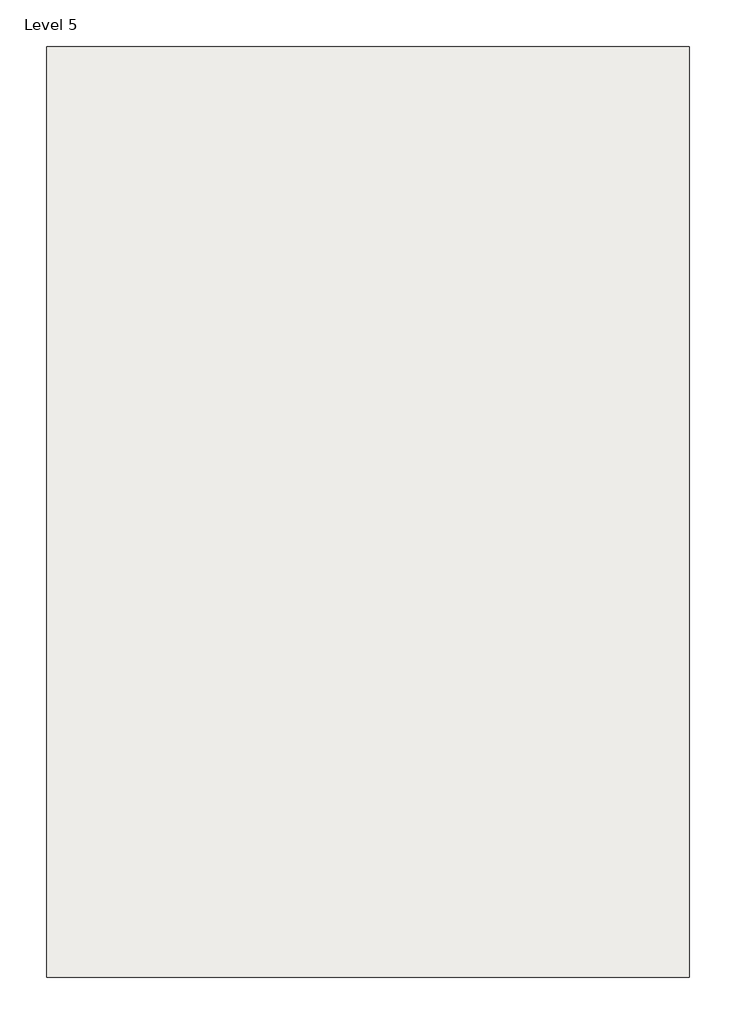
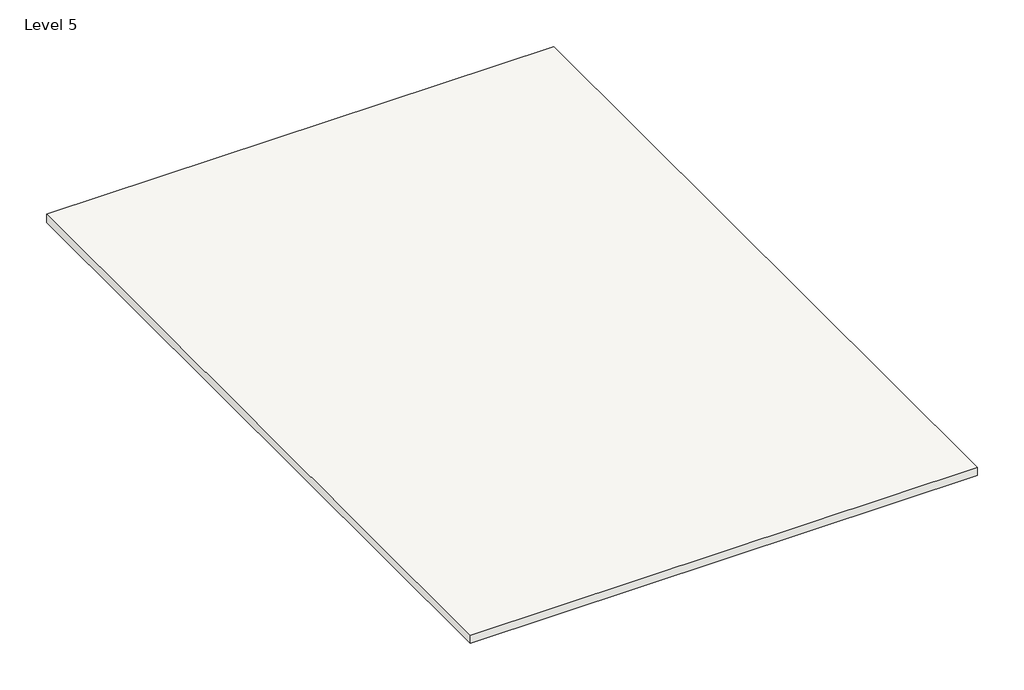
# One storey, incomplete: 1 roof.
"""IFC4 building model written with IfcOpenShell, lengths in millimetres."""

from ifc_helpers import new_model, si_unit, frame, origin, place, context, project, spatial, polyline, outline, extrude, element, save

model = new_model("IFC4")

# Units and contexts
model_context = context("Model", 3, world=origin())
ifc_project = project(units=[si_unit("LENGTHUNIT", "METRE", prefix="MILLI")], contexts=[model_context])

# Site, building, storey
site = spatial("IfcSite", under=ifc_project)
building = spatial("IfcBuilding", under=site)
storey = spatial("IfcBuildingStorey", under=building, Name="Level 5", Elevation=9601.2)

# Roof
placement = place(None, origin())
element("IfcRoof", 1, ObjectType="Generic - 12\"", at=placement, inside=storey, context=model_context, shape_type="SweptSolid", body=[
    extrude(outline(polyline([(-5674.8415084, 6938.9935985), (3164.3584916, 6938.9935985), (3164.3584916, -5862.6064015), (-5674.8415084, -5862.6064015), (-5674.8415084, 6938.9935985)])), frame((0.0, 0.0, 9448.8), z_axis=(0.0, 0.0, 1.0), x_axis=(1.0, 0.0, 0.0)), (0.0, 0.0, 1.0), 152.4),
])

save(model, "model.ifc")

# Revit data of these elements
# Type "Generic - 12\""
#   Assembly Code = "B1020"
#   Layers, outside or top first: 0' - 6" no material (function 1)
# Element 1 (IfcRoof, "Generic - 12\"")
#   built-in parameter 1001705 = 31.5 (stored number, unit not read)
#   built-in parameter 1001701 = -0.5 (stored number, unit not read)
#   built-in parameter 1001710 = 33615
#   Phase Created = New Construction
#   Materials on its faces: "Default Roof"
# Materials
#   "Default Roof": colour RGB 88 101 114, transparency 0, Cost = 0
